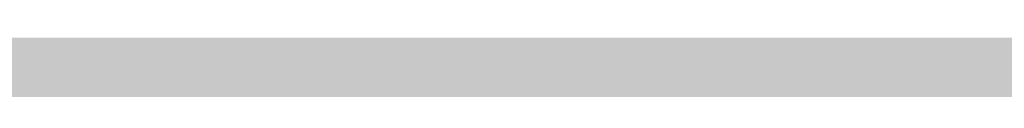
# Model space of a CAD drawing. Units: feet. Extents: x 3168 to 4724, y 827 to 1477.
# Tile 2 of 256: x 3231.95 to 3244.72, y 1098.34 to 1099. Entities that reach past the tile are written whole.
import ezdxf

# ---------------------------------------------------------------- set-up
doc = ezdxf.new("R2010")
doc.units = ezdxf.units.FT
doc.layers.add('A-ELEV', color=7, linetype='Continuous', lineweight=35)
doc.layers.add('A-ELEV-PATT', color=8, linetype='Continuous', lineweight=13)

msp = doc.modelspace()

# ---------------------------------------------------------------- hatches: boundary and pattern name
at = {"layer": 'A-ELEV-PATT'}
h = msp.add_hatch(color=256, dxfattribs=at)
h.dxf.hatch_style = 1
h.paths.add_polyline_path([(3384.525, 1099.016), (3335.029, 1099.016), (3299.317, 1099.016), (3273.143, 1099.016), (3217.565, 1099.016), (3168.069, 827.116), (3335.029, 827.116)])

# ---------------------------------------------------------------- linework, layer by layer
at = {"layer": 'A-ELEV'}
msp.add_open_spline([(3808.52, 1099.016), (3808.52, 1141.413), (3808.52, 1183.81), (3808.52, 1226.635), (3808.52, 1227.064), (3808.52, 1227.492), (3811.492, 1248.995), (3814.464, 1270.498), (3817.465, 1292.218), (3817.495, 1292.435), (3817.525, 1292.652), (3817.573, 1310.107), (3817.62, 1327.562), (3817.668, 1345.016), (3817.668, 1345.458), (3817.668, 1345.9), (3817.668, 1346.456), (3817.668, 1346.571), (3817.668, 1346.753), (3817.668, 1346.82), (3817.668, 1346.935), (3817.668, 1346.982), (3817.668, 1347.039), (3817.668, 1347.047), (3817.668, 1347.074), (3817.668, 1347.059), (3817.668, 1347.062), (3817.668, 1347.063), (3817.668, 1347.066), (3817.668, 1347.068), (3817.668, 1347.075), (3817.668, 1347.079), (3817.668, 1347.093), (3817.668, 1347.102), (3817.668, 1347.129), (3817.668, 1347.147), (3817.667, 1347.2), (3817.667, 1347.236), (3817.666, 1347.343), (3817.665, 1347.415), (3817.661, 1347.628), (3817.657, 1347.77), (3817.64, 1348.192), (3817.624, 1348.472), (3817.559, 1349.3), (3817.496, 1349.841), (3817.255, 1351.424), (3817.026, 1352.429), (3816.307, 1354.889), (3815.744, 1356.269), (3814.464, 1358.819), (3813.746, 1359.991), (3812.196, 1362.172), (3811.362, 1363.182), (3809.589, 1365.069), (3808.649, 1365.946), (3806.654, 1367.58), (3805.6, 1368.336), (3803.353, 1369.722), (3802.161, 1370.352), (3799.601, 1371.454), (3798.233, 1371.925), (3795.28, 1372.635), (3793.693, 1372.872), (3791.869, 1372.926), (3791.741, 1372.929), (3791.353, 1372.934), (3791.093, 1372.933), (3790.304, 1372.915), (3789.77, 1372.884), (3789.209, 1372.83), (3789.191, 1372.828), (3789.135, 1372.823), (3789.098, 1372.819), (3789.048, 1372.814), (3789.036, 1372.813), (3789, 1372.809), (3788.976, 1372.806), (3788.949, 1372.803), (3788.947, 1372.803), (3788.943, 1372.803), (3788.941, 1372.802), (3788.939, 1372.802), (3788.938, 1372.802), (3788.935, 1372.802), (3788.868, 1372.794), (3788.757, 1372.782), (3788.702, 1372.776), (3788.536, 1372.758), (3788.425, 1372.746), (3788.093, 1372.709), (3787.872, 1372.685), (3787.208, 1372.612), (3786.765, 1372.563), (3785.437, 1372.417), (3784.551, 1372.32), (3781.895, 1372.027), (3780.125, 1371.833), (3774.813, 1371.248), (3771.271, 1370.859), (3760.647, 1369.69), (3753.564, 1368.911), (3732.316, 1366.573), (3718.15, 1365.015), (3694.007, 1362.359), (3684.029, 1361.262), (3674.051, 1360.164), (3664.601, 1360.164), (3655.151, 1360.164), (3626.801, 1360.164), (3607.901, 1360.164), (3551.202, 1360.164), (3513.402, 1360.164), (3467.725, 1360.164), (3459.848, 1360.164), (3436.215, 1360.164), (3420.46, 1360.164), (3373.194, 1360.164), (3341.684, 1360.164), (3302.848, 1360.164), (3295.523, 1360.164), (3286.038, 1360.164), (3283.879, 1360.164), (3277.403, 1360.164), (3273.085, 1360.164), (3267.733, 1360.164), (3266.699, 1360.164), (3263.597, 1360.164), (3261.528, 1360.164), (3259.237, 1360.164), (3259.014, 1360.164), (3258.344, 1360.164), (3257.897, 1360.164), (3257.431, 1360.164), (3257.411, 1360.164), (3257.371, 1360.164), (3257.375, 1360.164), (3257.375, 1360.164), (3257.374, 1360.164), (3257.372, 1360.164), (3257.371, 1360.164), (3257.367, 1360.164), (3257.364, 1360.164), (3257.356, 1360.164), (3257.351, 1360.164), (3257.335, 1360.164), (3257.324, 1360.164), (3257.293, 1360.164), (3257.272, 1360.164), (3257.208, 1360.163), (3257.166, 1360.163), (3257.04, 1360.161), (3256.956, 1360.16), (3256.706, 1360.153), (3256.539, 1360.147), (3256.044, 1360.122), (3255.717, 1360.097), (3254.752, 1360), (3254.128, 1359.907), (3252.18, 1359.525), (3250.942, 1359.144), (3248.67, 1358.243), (3247.636, 1357.724), (3245.733, 1356.603), (3244.863, 1356.002), (3243.253, 1354.743), (3242.512, 1354.085), (3240.751, 1352.345), (3239.801, 1351.23), (3238.088, 1348.872), (3237.325, 1347.63), (3235.983, 1344.972), (3235.402, 1343.555), (3234.591, 1340.815), (3234.311, 1339.544), (3233.976, 1336.803), (3233.922, 1335.331), (3234.149, 1332.591), (3234.35, 1331.367), (3234.72, 1329.999), (3234.752, 1329.883), (3234.854, 1329.535), (3234.926, 1329.302), (3235.025, 1329.003), (3235.047, 1328.937), (3235.078, 1328.847), (3235.086, 1328.823), (3235.111, 1328.751), (3235.128, 1328.703), (3235.148, 1328.646), (3235.151, 1328.638), (3235.156, 1328.624), (3235.158, 1328.618), (3235.16, 1328.612), (3235.166, 1328.597), (3235.18, 1328.556), (3235.19, 1328.528), (3235.221, 1328.443), (3235.241, 1328.386), (3235.302, 1328.216), (3235.343, 1328.102), (3235.465, 1327.762), (3235.546, 1327.535), (3235.79, 1326.853), (3235.953, 1326.399), (3236.44, 1325.037), (3236.766, 1324.128), (3237.741, 1321.403), (3238.392, 1319.587), (3240.344, 1314.137), (3241.645, 1310.504), (3245.548, 1299.604), (3248.15, 1292.337), (3255.956, 1270.537), (3261.16, 1256.004), (3267.388, 1238.612), (3268.411, 1235.753), (3269.51, 1232.684), (3269.586, 1232.474), (3269.707, 1232.136), (3269.752, 1232.008), (3269.827, 1231.799), (3269.856, 1231.718), (3269.906, 1231.578), (3269.927, 1231.52), (3269.972, 1231.393), (3269.997, 1231.325), (3270.027, 1231.243), (3270.032, 1231.228), (3270.04, 1231.204), (3270.039, 1231.207), (3270.039, 1231.207), (3270.039, 1231.206), (3270.04, 1231.206), (3270.04, 1231.205), (3270.04, 1231.204), (3270.04, 1231.204), (3270.041, 1231.201), (3270.042, 1231.2), (3270.043, 1231.195), (3270.045, 1231.192), (3270.048, 1231.183), (3270.05, 1231.177), (3270.056, 1231.159), (3270.061, 1231.147), (3270.074, 1231.111), (3270.083, 1231.087), (3270.109, 1231.014), (3270.127, 1230.966), (3270.18, 1230.822), (3270.216, 1230.727), (3270.325, 1230.442), (3270.4, 1230.253), (3270.629, 1229.691), (3270.789, 1229.324), (3271.286, 1228.238), (3271.643, 1227.54), (3272.776, 1225.515), (3273.614, 1224.261), (3275.416, 1221.918), (3276.38, 1220.829), (3278.897, 1218.318), (3280.512, 1216.98), (3283.951, 1214.603), (3285.776, 1213.564), (3289.654, 1211.813), (3291.707, 1211.101), (3294.03, 1210.574), (3294.169, 1210.543), (3294.588, 1210.454), (3294.869, 1210.399), (3295.718, 1210.243), (3296.293, 1210.155), (3296.979, 1210.07), (3297.083, 1210.058), (3297.393, 1210.023), (3297.602, 1210.002), (3298.229, 1209.946), (3298.652, 1209.917), (3299.13, 1209.895), (3299.181, 1209.893), (3299.334, 1209.887), (3299.437, 1209.883), (3299.745, 1209.874), (3299.951, 1209.871), (3300.195, 1209.869), (3300.232, 1209.869), (3300.28, 1209.869), (3300.291, 1209.869), (3300.306, 1209.869), (3300.311, 1209.869), (3300.321, 1209.869), (3300.326, 1209.869), (3300.332, 1209.869), (3300.334, 1209.869), (3300.337, 1209.869), (3300.338, 1209.869), (3300.341, 1209.869), (3300.343, 1209.869), (3300.346, 1209.869), (3300.346, 1209.869), (3300.346, 1209.869), (3300.366, 1209.869), (3300.388, 1209.869), (3300.399, 1209.869), (3300.431, 1209.869), (3300.453, 1209.869), (3300.517, 1209.869), (3300.561, 1209.869), (3300.69, 1209.869), (3300.777, 1209.869), (3301.036, 1209.869), (3301.209, 1209.869), (3301.727, 1209.869), (3302.073, 1209.869), (3303.11, 1209.869), (3303.801, 1209.869), (3305.875, 1209.869), (3307.257, 1209.869), (3311.405, 1209.869), (3314.17, 1209.869), (3322.466, 1209.869), (3327.996, 1209.869), (3344.586, 1209.869), (3355.647, 1209.869), (3388.828, 1209.869), (3410.949, 1209.869), (3477.312, 1209.869), (3521.554, 1209.869), (3566.836, 1209.869), (3567.877, 1209.869), (3570.999, 1209.869), (3573.08, 1209.869), (3575.781, 1209.869), (3576.401, 1209.869), (3577.296, 1209.869), (3577.571, 1209.869), (3578.397, 1209.869), (3578.948, 1209.869), (3579.756, 1209.869), (3580.015, 1209.869), (3580.343, 1209.869), (3580.327, 1209.869), (3580.327, 1209.869), (3580.327, 1209.869), (3580.328, 1209.869), (3580.328, 1209.869), (3580.329, 1209.869), (3580.33, 1209.869), (3580.331, 1209.869), (3580.333, 1209.869), (3580.336, 1209.869), (3580.339, 1209.869), (3580.346, 1209.869), (3580.351, 1209.869), (3580.366, 1209.869), (3580.375, 1209.869), (3580.405, 1209.868), (3580.424, 1209.868), (3580.483, 1209.868), (3580.522, 1209.868), (3580.64, 1209.867), (3580.719, 1209.865), (3580.956, 1209.861), (3581.115, 1209.856), (3581.594, 1209.837), (3581.916, 1209.818), (3582.89, 1209.742), (3583.548, 1209.666), (3585.532, 1209.361), (3586.867, 1209.054), (3589.472, 1208.252), (3590.74, 1207.758), (3591.995, 1207.159), (3592.058, 1207.129), (3592.244, 1207.038), (3592.368, 1206.977), (3592.735, 1206.79), (3592.977, 1206.663), (3593.245, 1206.516), (3593.275, 1206.5), (3593.365, 1206.45), (3593.425, 1206.416), (3593.604, 1206.315), (3593.723, 1206.247), (3593.857, 1206.168), (3593.874, 1206.158), (3593.926, 1206.128), (3593.96, 1206.108), (3594.062, 1206.047), (3594.13, 1206.006), (3594.208, 1205.958), (3594.22, 1205.951), (3594.253, 1205.931), (3594.276, 1205.917), (3594.343, 1205.876), (3594.388, 1205.848), (3594.434, 1205.819), (3594.435, 1205.818), (3594.44, 1205.815), (3594.443, 1205.813), (3594.447, 1205.811), (3594.448, 1205.81), (3594.449, 1205.81), (3594.449, 1205.809), (3594.45, 1205.809), (3594.45, 1205.808), (3594.451, 1205.808), (3594.467, 1205.798), (3594.493, 1205.782), (3594.506, 1205.774), (3594.545, 1205.749), (3594.571, 1205.733), (3594.648, 1205.684), (3594.7, 1205.652), (3594.855, 1205.555), (3594.959, 1205.49), (3595.269, 1205.295), (3595.476, 1205.166), (3596.097, 1204.776), (3596.511, 1204.517), (3597.753, 1203.739), (3598.581, 1203.22), (3601.064, 1201.664), (3602.72, 1200.626), (3607.687, 1197.513), (3610.998, 1195.438), (3620.932, 1189.212), (3627.555, 1185.061), (3647.423, 1172.61), (3660.668, 1164.309), (3700.403, 1139.405), (3726.894, 1122.803), (3757.206, 1103.806), (3761.027, 1101.411), (3764.848, 1099.016), (3745.328, 1099.016), (3725.808, 1099.016), (3706.288, 1099.016), (3706.288, 1108.453), (3706.288, 1117.89), (3706.288, 1127.327), (3710.751, 1127.327), (3715.213, 1127.327), (3719.676, 1127.327)], degree=3, knots=[0, 0, 0, 0, 0.982037, 0.982037, 0.991957, 0.991957, 0.991957, 1.966522, 1.966522, 1.976367, 1.976367, 1.976367, 2.976367, 2.976367, 2.976367, 3.00169, 3.00169, 3.008272, 3.008272, 3.012129, 3.012129, 3.014851, 3.014851, 3.015353, 3.015353, 3.016359, 3.016359, 3.017365, 3.017365, 3.019376, 3.019376, 3.023398, 3.023398, 3.031442, 3.031442, 3.047531, 3.047531, 3.079708, 3.079708, 3.144063, 3.144063, 3.272772, 3.272772, 3.53019, 3.53019, 4.045026, 4.045026, 5.074698, 5.074698, 6.700878, 6.700878, 8.327058, 8.327058, 9.953238, 9.953238, 11.579418, 11.579418, 13.205598, 13.205598, 14.831778, 14.831778, 16.457958, 16.457958, 18.084138, 18.084138, 18.206872, 18.206872, 18.45234, 18.45234, 18.943275, 18.943275, 18.960093, 18.960093, 18.993729, 18.993729, 19.00461, 19.00461, 19.026374, 19.026374, 19.028737, 19.028737, 19.03018, 19.03018, 19.030897, 19.030897, 19.032332, 19.032332, 19.033766, 19.033766, 19.036636, 19.036636, 19.042374, 19.042374, 19.053851, 19.053851, 19.076805, 19.076805, 19.122714, 19.122714, 19.21453, 19.21453, 19.398163, 19.398163, 19.765429, 19.765429, 20.024128, 20.024128, 20.024128, 20.092031, 20.092031, 20.227836, 20.227836, 20.499446, 20.499446, 20.556051, 20.556051, 20.66926, 20.66926, 20.895678, 20.895678, 20.948316, 20.948316, 20.963829, 20.963829, 20.994855, 20.994855, 21.002285, 21.002285, 21.017146, 21.017146, 21.01875, 21.01875, 21.021959, 21.021959, 21.022102, 21.022102, 21.022249, 21.022249, 21.022708, 21.022708, 21.023627, 21.023627, 21.025464, 21.025464, 21.029138, 21.029138, 21.036486, 21.036486, 21.051183, 21.051183, 21.080575, 21.080575, 21.139361, 21.139361, 21.256932, 21.256932, 21.492073, 21.492073, 21.962356, 21.962356, 23.01002, 23.01002, 24.057684, 24.057684, 25.105348, 25.105348, 26.153011, 26.153011, 27.776787, 27.776787, 29.400562, 29.400562, 31.024337, 31.024337, 32.278801, 32.278801, 33.533265, 33.533265, 34.467568, 34.467568, 34.553971, 34.553971, 34.726776, 34.726776, 34.775309, 34.775309, 34.793079, 34.793079, 34.82862, 34.82862, 34.834979, 34.834979, 34.839039, 34.839039, 34.839411, 34.839411, 34.840285, 34.840285, 34.842034, 34.842034, 34.845531, 34.845531, 34.852525, 34.852525, 34.866512, 34.866512, 34.894488, 34.894488, 34.950439, 34.950439, 35.062342, 35.062342, 35.286147, 35.286147, 35.733758, 35.733758, 35.821815, 35.821815, 35.828283, 35.828283, 35.832225, 35.832225, 35.834724, 35.834724, 35.836521, 35.836521, 35.838617, 35.838617, 35.839073, 35.839073, 35.839345, 35.839345, 35.839617, 35.839617, 35.840161, 35.840161, 35.841249, 35.841249, 35.843425, 35.843425, 35.847778, 35.847778, 35.856482, 35.856482, 35.873891, 35.873891, 35.908709, 35.908709, 35.978345, 35.978345, 36.117617, 36.117617, 36.396161, 36.396161, 36.953248, 36.953248, 38.067423, 38.067423, 40.295772, 40.295772, 42.524122, 42.524122, 45.81453, 45.81453, 49.104937, 49.104937, 52.395345, 52.395345, 52.603776, 52.603776, 53.020639, 53.020639, 53.854363, 53.854363, 54.001655, 54.001655, 54.296238, 54.296238, 54.885405, 54.885405, 54.955785, 54.955785, 55.096546, 55.096546, 55.378067, 55.378067, 55.42849, 55.42849, 55.442691, 55.442691, 55.449436, 55.449436, 55.455957, 55.455957, 55.458409, 55.458409, 55.459872, 55.459872, 55.462798, 55.462798, 55.462856, 55.462856, 55.462972, 55.462972, 55.463088, 55.463088, 55.463319, 55.463319, 55.463782, 55.463782, 55.464708, 55.464708, 55.46656, 55.46656, 55.470263, 55.470263, 55.47767, 55.47767, 55.492484, 55.492484, 55.522112, 55.522112, 55.581369, 55.581369, 55.699882, 55.699882, 55.936907, 55.936907, 56.410959, 56.410959, 56.42211, 56.42211, 56.444413, 56.444413, 56.451051, 56.451051, 56.454001, 56.454001, 56.459901, 56.459901, 56.462666, 56.462666, 56.463418, 56.463418, 56.464171, 56.464171, 56.465675, 56.465675, 56.468684, 56.468684, 56.474702, 56.474702, 56.486738, 56.486738, 56.51081, 56.51081, 56.558955, 56.558955, 56.655243, 56.655243, 56.847821, 56.847821, 57.232975, 57.232975, 58.003284, 58.003284, 59.543901, 59.543901, 62.625137, 62.625137, 68.787607, 68.787607, 74.950078, 74.950078, 75.27336, 75.27336, 75.919923, 75.919923, 77.213051, 77.213051, 77.377769, 77.377769, 77.707206, 77.707206, 78.366079, 78.366079, 78.462532, 78.462532, 78.655436, 78.655436, 79.041245, 79.041245, 79.105735, 79.105735, 79.234714, 79.234714, 79.492672, 79.492672, 79.502197, 79.502197, 79.521249, 79.521249, 79.523534, 79.523534, 79.528103, 79.528103, 79.528682, 79.528682, 79.528885, 79.528885, 79.529089, 79.529089, 79.529495, 79.529495, 79.530308, 79.530308, 79.531935, 79.531935, 79.535187, 79.535187, 79.541693, 79.541693, 79.554704, 79.554704, 79.580725, 79.580725, 79.632769, 79.632769, 79.736856, 79.736856, 79.94503, 79.94503, 80.361377, 80.361377, 80.421435, 80.421435, 80.421435, 81.421435, 81.421435, 81.421435, 82.421435, 82.421435, 82.421435, 83.421435, 83.421435, 83.421435, 83.421435], dxfattribs=at)

doc.saveas('drawing.dxf')
